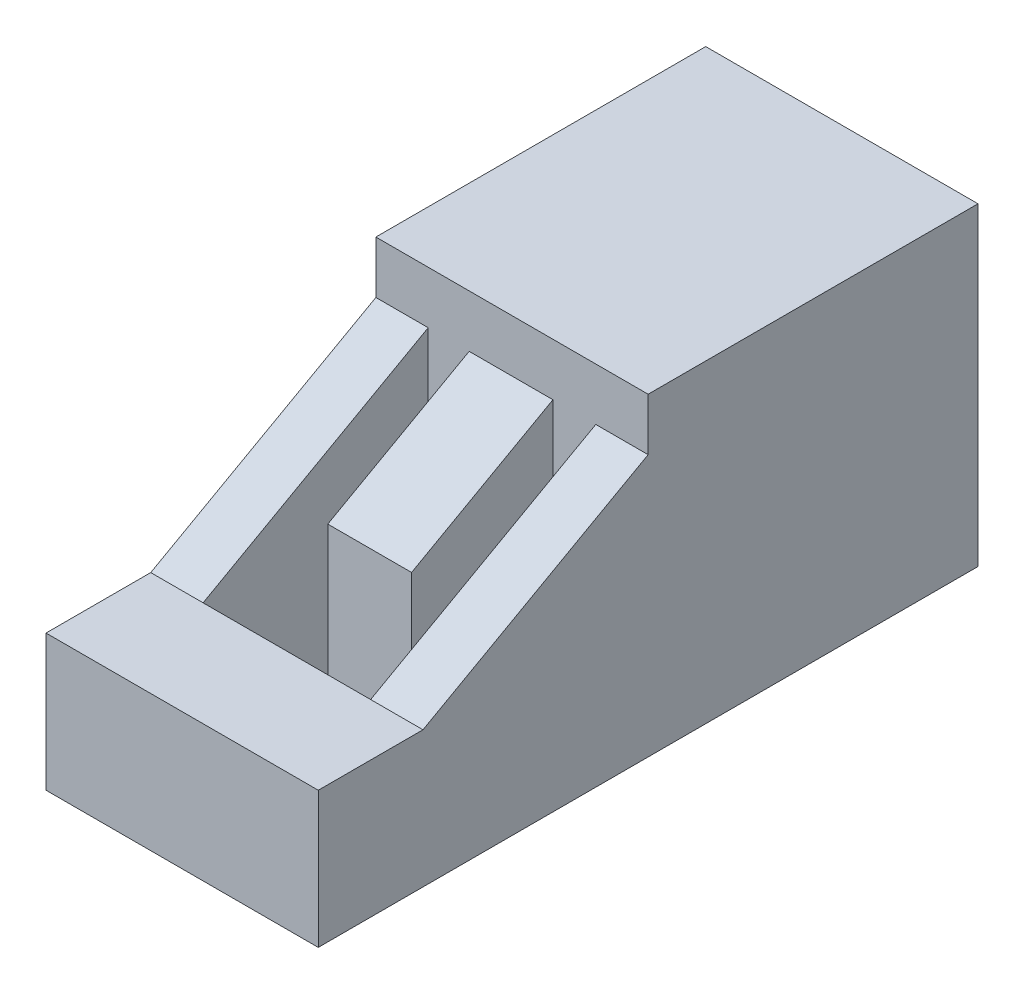
ISO-10303-21;
HEADER;
FILE_DESCRIPTION(('STEP AP214'),'2;1');
FILE_NAME('part.step','',(''),(''),'','','');
FILE_SCHEMA(('AUTOMOTIVE_DESIGN { 1 0 10303 214 1 1 1 1 }'));
ENDSEC;
DATA;
#1=APPLICATION_CONTEXT('core data for automotive mechanical design processes');
#2=APPLICATION_PROTOCOL_DEFINITION('international standard','automotive_design',2000,#1);
#3=PRODUCT_CONTEXT('',#1,'mechanical');
#4=PRODUCT('Part','Part','',(#3));
#5=PRODUCT_RELATED_PRODUCT_CATEGORY('part','',(#4));
#6=PRODUCT_DEFINITION_FORMATION('','',#4);
#7=PRODUCT_DEFINITION_CONTEXT('part definition',#1,'design');
#8=PRODUCT_DEFINITION('design','',#6,#7);
#9=PRODUCT_DEFINITION_SHAPE('','',#8);
#10=(LENGTH_UNIT() NAMED_UNIT(*) SI_UNIT(.MILLI.,.METRE.));
#11=(NAMED_UNIT(*) PLANE_ANGLE_UNIT() SI_UNIT($,.RADIAN.));
#12=(NAMED_UNIT(*) SI_UNIT($,.STERADIAN.) SOLID_ANGLE_UNIT());
#13=UNCERTAINTY_MEASURE_WITH_UNIT(LENGTH_MEASURE(1.E-05),#10,'distance_accuracy_value','');
#14=(GEOMETRIC_REPRESENTATION_CONTEXT(3) GLOBAL_UNCERTAINTY_ASSIGNED_CONTEXT((#13)) GLOBAL_UNIT_ASSIGNED_CONTEXT((#10,
#11,#12)) REPRESENTATION_CONTEXT('',''));
#15=CARTESIAN_POINT('',(0.,0.,0.));
#16=DIRECTION('',(0.,0.,1.));
#17=DIRECTION('',(1.,0.,0.));
#18=AXIS2_PLACEMENT_3D('',#15,#16,#17);
#19=CARTESIAN_POINT('',(26.,-15.,31.5));
#20=DIRECTION('',(0.,1.,0.));
#21=DIRECTION('',(0.,0.,1.));
#22=AXIS2_PLACEMENT_3D('',#19,#20,#21);
#23=PLANE('',#22);
#24=DIRECTION('',(0.,0.,1.));
#25=VECTOR('',#24,1.);
#26=CARTESIAN_POINT('',(8.90839032863548,-15.,31.5));
#27=LINE('',#26,#25);
#28=CARTESIAN_POINT('',(8.90839032863548,-15.,0.));
#29=VERTEX_POINT('',#28);
#30=CARTESIAN_POINT('',(8.90839032863548,-15.,13.5));
#31=VERTEX_POINT('',#30);
#32=EDGE_CURVE('E171',#29,#31,#27,.T.);
#33=ORIENTED_EDGE('',*,*,#32,.F.);
#34=DIRECTION('',(1.,0.,0.));
#35=VECTOR('',#34,1.);
#36=CARTESIAN_POINT('',(26.,-15.,0.));
#37=LINE('',#36,#35);
#38=CARTESIAN_POINT('',(4.99999999999999,-15.,0.));
#39=VERTEX_POINT('',#38);
#40=EDGE_CURVE('E180',#39,#29,#37,.T.);
#41=ORIENTED_EDGE('',*,*,#40,.F.);
#42=DIRECTION('',(0.,0.,1.));
#43=VECTOR('',#42,1.);
#44=CARTESIAN_POINT('',(4.99999999999999,-15.,31.5));
#45=LINE('',#44,#43);
#46=CARTESIAN_POINT('',(4.99999999999999,-15.,21.5));
#47=VERTEX_POINT('',#46);
#48=EDGE_CURVE('E179',#39,#47,#45,.T.);
#49=ORIENTED_EDGE('',*,*,#48,.T.);
#50=DIRECTION('',(1.,0.,0.));
#51=VECTOR('',#50,1.);
#52=CARTESIAN_POINT('',(26.,-15.,21.5));
#53=LINE('',#52,#51);
#54=CARTESIAN_POINT('',(21.,-15.,21.5));
#55=VERTEX_POINT('',#54);
#56=EDGE_CURVE('E185',#47,#55,#53,.T.);
#57=ORIENTED_EDGE('',*,*,#56,.T.);
#58=DIRECTION('',(0.,0.,1.));
#59=VECTOR('',#58,1.);
#60=CARTESIAN_POINT('',(21.,-15.,31.5));
#61=LINE('',#60,#59);
#62=CARTESIAN_POINT('',(21.,-15.,0.));
#63=VERTEX_POINT('',#62);
#64=EDGE_CURVE('E183',#63,#55,#61,.T.);
#65=ORIENTED_EDGE('',*,*,#64,.F.);
#66=DIRECTION('',(1.,0.,0.));
#67=VECTOR('',#66,1.);
#68=CARTESIAN_POINT('',(26.,-15.,0.));
#69=LINE('',#68,#67);
#70=CARTESIAN_POINT('',(16.9083903286355,-15.,0.));
#71=VERTEX_POINT('',#70);
#72=EDGE_CURVE('E190',#71,#63,#69,.T.);
#73=ORIENTED_EDGE('',*,*,#72,.F.);
#74=DIRECTION('',(0.,0.,1.));
#75=VECTOR('',#74,1.);
#76=CARTESIAN_POINT('',(16.9083903286355,-15.,31.5));
#77=LINE('',#76,#75);
#78=CARTESIAN_POINT('',(16.9083903286355,-15.,13.5));
#79=VERTEX_POINT('',#78);
#80=EDGE_CURVE('E163',#71,#79,#77,.T.);
#81=ORIENTED_EDGE('',*,*,#80,.T.);
#82=DIRECTION('',(1.,0.,0.));
#83=VECTOR('',#82,1.);
#84=CARTESIAN_POINT('',(26.,-15.,13.5));
#85=LINE('',#84,#83);
#86=EDGE_CURVE('E175',#31,#79,#85,.T.);
#87=ORIENTED_EDGE('',*,*,#86,.F.);
#88=EDGE_LOOP('',(#33,#41,#49,#57,#65,#73,#81,#87));
#89=FACE_BOUND('',#88,.T.);
#90=DIRECTION('',(0.,0.,-1.));
#91=VECTOR('',#90,1.);
#92=CARTESIAN_POINT('',(0.,-15.,31.5));
#93=LINE('',#92,#91);
#94=CARTESIAN_POINT('',(0.,-15.,31.5));
#95=VERTEX_POINT('',#94);
#96=CARTESIAN_POINT('',(0.,-15.,-31.5));
#97=VERTEX_POINT('',#96);
#98=EDGE_CURVE('E224',#95,#97,#93,.T.);
#99=ORIENTED_EDGE('',*,*,#98,.T.);
#100=DIRECTION('',(-1.,0.,0.));
#101=VECTOR('',#100,1.);
#102=CARTESIAN_POINT('',(26.,-15.,-31.5));
#103=LINE('',#102,#101);
#104=CARTESIAN_POINT('',(26.,-15.,-31.5));
#105=VERTEX_POINT('',#104);
#106=EDGE_CURVE('E226',#105,#97,#103,.T.);
#107=ORIENTED_EDGE('',*,*,#106,.F.);
#108=DIRECTION('',(0.,0.,-1.));
#109=VECTOR('',#108,1.);
#110=CARTESIAN_POINT('',(26.,-15.,31.5));
#111=LINE('',#110,#109);
#112=CARTESIAN_POINT('',(26.,-15.,31.5));
#113=VERTEX_POINT('',#112);
#114=EDGE_CURVE('E228',#113,#105,#111,.T.);
#115=ORIENTED_EDGE('',*,*,#114,.F.);
#116=DIRECTION('',(-1.,0.,0.));
#117=VECTOR('',#116,1.);
#118=CARTESIAN_POINT('',(26.,-15.,31.5));
#119=LINE('',#118,#117);
#120=EDGE_CURVE('E242',#113,#95,#119,.T.);
#121=ORIENTED_EDGE('',*,*,#120,.T.);
#122=EDGE_LOOP('',(#99,#107,#115,#121));
#123=FACE_BOUND('',#122,.T.);
#124=ADVANCED_FACE('F41',(#89,#123),#23,.F.);
#125=CARTESIAN_POINT('',(0.,7.62474226804124,4.25567010309278));
#126=DIRECTION('',(0.,-0.873197702014912,-0.487366159264137));
#127=DIRECTION('',(0.,0.487366159264137,-0.873197702014913));
#128=AXIS2_PLACEMENT_3D('',#125,#126,#127);
#129=PLANE('',#128);
#130=DIRECTION('',(0.,0.487366159264137,-0.873197702014913));
#131=VECTOR('',#130,1.);
#132=CARTESIAN_POINT('',(21.,7.62474226804124,4.25567010309278));
#133=LINE('',#132,#131);
#134=CARTESIAN_POINT('',(21.,-2.,21.5));
#135=VERTEX_POINT('',#134);
#136=CARTESIAN_POINT('',(21.,9.99999999999999,0.));
#137=VERTEX_POINT('',#136);
#138=EDGE_CURVE('E11',#135,#137,#133,.T.);
#139=ORIENTED_EDGE('',*,*,#138,.F.);
#140=DIRECTION('',(1.,0.,0.));
#141=VECTOR('',#140,1.);
#142=CARTESIAN_POINT('',(0.,-2.,21.5));
#143=LINE('',#142,#141);
#144=CARTESIAN_POINT('',(26.,-2.,21.5));
#145=VERTEX_POINT('',#144);
#146=EDGE_CURVE('E200',#135,#145,#143,.T.);
#147=ORIENTED_EDGE('',*,*,#146,.T.);
#148=DIRECTION('',(0.,0.487366159264137,-0.873197702014912));
#149=VECTOR('',#148,1.);
#150=CARTESIAN_POINT('',(26.,7.62474226804124,4.25567010309278));
#151=LINE('',#150,#149);
#152=CARTESIAN_POINT('',(26.,10.,0.));
#153=VERTEX_POINT('',#152);
#154=EDGE_CURVE('E205',#145,#153,#151,.T.);
#155=ORIENTED_EDGE('',*,*,#154,.T.);
#156=DIRECTION('',(1.,0.,0.));
#157=VECTOR('',#156,1.);
#158=CARTESIAN_POINT('',(0.,10.,0.));
#159=LINE('',#158,#157);
#160=EDGE_CURVE('E212',#137,#153,#159,.T.);
#161=ORIENTED_EDGE('',*,*,#160,.F.);
#162=EDGE_LOOP('',(#139,#147,#155,#161));
#163=FACE_BOUND('',#162,.T.);
#164=ADVANCED_FACE('F286',(#163),#129,.F.);
#165=CARTESIAN_POINT('',(26.,15.,-31.5));
#166=DIRECTION('',(0.,0.,1.));
#167=DIRECTION('',(1.,0.,0.));
#168=AXIS2_PLACEMENT_3D('',#165,#166,#167);
#169=PLANE('',#168);
#170=DIRECTION('',(0.,1.,0.));
#171=VECTOR('',#170,1.);
#172=CARTESIAN_POINT('',(0.,15.,-31.5));
#173=LINE('',#172,#171);
#174=CARTESIAN_POINT('',(0.,15.,-31.5));
#175=VERTEX_POINT('',#174);
#176=EDGE_CURVE('E208',#97,#175,#173,.T.);
#177=ORIENTED_EDGE('',*,*,#176,.T.);
#178=DIRECTION('',(-1.,0.,0.));
#179=VECTOR('',#178,1.);
#180=CARTESIAN_POINT('',(26.,15.,-31.5));
#181=LINE('',#180,#179);
#182=CARTESIAN_POINT('',(26.,15.,-31.5));
#183=VERTEX_POINT('',#182);
#184=EDGE_CURVE('E244',#183,#175,#181,.T.);
#185=ORIENTED_EDGE('',*,*,#184,.F.);
#186=DIRECTION('',(0.,1.,0.));
#187=VECTOR('',#186,1.);
#188=CARTESIAN_POINT('',(26.,15.,-31.5));
#189=LINE('',#188,#187);
#190=EDGE_CURVE('E218',#105,#183,#189,.T.);
#191=ORIENTED_EDGE('',*,*,#190,.F.);
#192=ORIENTED_EDGE('',*,*,#106,.T.);
#193=EDGE_LOOP('',(#177,#185,#191,#192));
#194=FACE_BOUND('',#193,.T.);
#195=ADVANCED_FACE('F43',(#194),#169,.F.);
#196=CARTESIAN_POINT('',(26.,15.,31.5));
#197=DIRECTION('',(0.,-1.,0.));
#198=DIRECTION('',(0.,0.,-1.));
#199=AXIS2_PLACEMENT_3D('',#196,#197,#198);
#200=PLANE('',#199);
#201=DIRECTION('',(1.,0.,0.));
#202=VECTOR('',#201,1.);
#203=CARTESIAN_POINT('',(0.,15.,0.));
#204=LINE('',#203,#202);
#205=CARTESIAN_POINT('',(0.,15.,0.));
#206=VERTEX_POINT('',#205);
#207=CARTESIAN_POINT('',(26.,15.,0.));
#208=VERTEX_POINT('',#207);
#209=EDGE_CURVE('E207',#206,#208,#204,.T.);
#210=ORIENTED_EDGE('',*,*,#209,.T.);
#211=DIRECTION('',(0.,0.,1.));
#212=VECTOR('',#211,1.);
#213=CARTESIAN_POINT('',(26.,15.,31.5));
#214=LINE('',#213,#212);
#215=EDGE_CURVE('E225',#183,#208,#214,.T.);
#216=ORIENTED_EDGE('',*,*,#215,.F.);
#217=ORIENTED_EDGE('',*,*,#184,.T.);
#218=DIRECTION('',(0.,0.,1.));
#219=VECTOR('',#218,1.);
#220=CARTESIAN_POINT('',(0.,15.,31.5));
#221=LINE('',#220,#219);
#222=EDGE_CURVE('E233',#175,#206,#221,.T.);
#223=ORIENTED_EDGE('',*,*,#222,.T.);
#224=EDGE_LOOP('',(#210,#216,#217,#223));
#225=FACE_BOUND('',#224,.T.);
#226=ADVANCED_FACE('F266',(#225),#200,.F.);
#227=CARTESIAN_POINT('',(26.,15.,31.5));
#228=DIRECTION('',(0.,0.,-1.));
#229=DIRECTION('',(0.,1.,0.));
#230=AXIS2_PLACEMENT_3D('',#227,#228,#229);
#231=PLANE('',#230);
#232=DIRECTION('',(0.,-1.,0.));
#233=VECTOR('',#232,1.);
#234=CARTESIAN_POINT('',(26.,15.,31.5));
#235=LINE('',#234,#233);
#236=CARTESIAN_POINT('',(26.,-2.,31.5));
#237=VERTEX_POINT('',#236);
#238=EDGE_CURVE('E227',#237,#113,#235,.T.);
#239=ORIENTED_EDGE('',*,*,#238,.F.);
#240=DIRECTION('',(1.,0.,0.));
#241=VECTOR('',#240,1.);
#242=CARTESIAN_POINT('',(0.,-2.,31.5));
#243=LINE('',#242,#241);
#244=CARTESIAN_POINT('',(0.,-2.,31.5));
#245=VERTEX_POINT('',#244);
#246=EDGE_CURVE('E206',#245,#237,#243,.T.);
#247=ORIENTED_EDGE('',*,*,#246,.F.);
#248=DIRECTION('',(0.,-1.,0.));
#249=VECTOR('',#248,1.);
#250=CARTESIAN_POINT('',(0.,15.,31.5));
#251=LINE('',#250,#249);
#252=EDGE_CURVE('E237',#245,#95,#251,.T.);
#253=ORIENTED_EDGE('',*,*,#252,.T.);
#254=ORIENTED_EDGE('',*,*,#120,.F.);
#255=EDGE_LOOP('',(#239,#247,#253,#254));
#256=FACE_BOUND('',#255,.T.);
#257=ADVANCED_FACE('F280',(#256),#231,.F.);
#258=CARTESIAN_POINT('',(26.,0.,0.));
#259=DIRECTION('',(1.,0.,0.));
#260=DIRECTION('',(0.,0.,-1.));
#261=AXIS2_PLACEMENT_3D('',#258,#259,#260);
#262=PLANE('',#261);
#263=DIRECTION('',(0.,0.,-1.));
#264=VECTOR('',#263,1.);
#265=CARTESIAN_POINT('',(26.,-2.,0.));
#266=LINE('',#265,#264);
#267=EDGE_CURVE('E189',#237,#145,#266,.T.);
#268=ORIENTED_EDGE('',*,*,#267,.F.);
#269=ORIENTED_EDGE('',*,*,#238,.T.);
#270=ORIENTED_EDGE('',*,*,#114,.T.);
#271=ORIENTED_EDGE('',*,*,#190,.T.);
#272=ORIENTED_EDGE('',*,*,#215,.T.);
#273=DIRECTION('',(0.,1.,0.));
#274=VECTOR('',#273,1.);
#275=CARTESIAN_POINT('',(26.,0.,0.));
#276=LINE('',#275,#274);
#277=EDGE_CURVE('E194',#153,#208,#276,.T.);
#278=ORIENTED_EDGE('',*,*,#277,.F.);
#279=ORIENTED_EDGE('',*,*,#154,.F.);
#280=EDGE_LOOP('',(#268,#269,#270,#271,#272,#278,#279));
#281=FACE_BOUND('',#280,.T.);
#282=ADVANCED_FACE('F281',(#281),#262,.T.);
#283=CARTESIAN_POINT('',(0.,0.,0.));
#284=DIRECTION('',(1.,0.,0.));
#285=DIRECTION('',(0.,0.,-1.));
#286=AXIS2_PLACEMENT_3D('',#283,#284,#285);
#287=PLANE('',#286);
#288=ORIENTED_EDGE('',*,*,#252,.F.);
#289=DIRECTION('',(0.,0.,-1.));
#290=VECTOR('',#289,1.);
#291=CARTESIAN_POINT('',(0.,-2.,0.));
#292=LINE('',#291,#290);
#293=CARTESIAN_POINT('',(0.,-2.,21.5));
#294=VERTEX_POINT('',#293);
#295=EDGE_CURVE('E186',#245,#294,#292,.T.);
#296=ORIENTED_EDGE('',*,*,#295,.T.);
#297=DIRECTION('',(0.,0.487366159264137,-0.873197702014912));
#298=VECTOR('',#297,1.);
#299=CARTESIAN_POINT('',(0.,7.62474226804124,4.25567010309278));
#300=LINE('',#299,#298);
#301=CARTESIAN_POINT('',(0.,10.,0.));
#302=VERTEX_POINT('',#301);
#303=EDGE_CURVE('E193',#294,#302,#300,.T.);
#304=ORIENTED_EDGE('',*,*,#303,.T.);
#305=DIRECTION('',(0.,1.,0.));
#306=VECTOR('',#305,1.);
#307=CARTESIAN_POINT('',(0.,0.,0.));
#308=LINE('',#307,#306);
#309=EDGE_CURVE('E198',#302,#206,#308,.T.);
#310=ORIENTED_EDGE('',*,*,#309,.T.);
#311=ORIENTED_EDGE('',*,*,#222,.F.);
#312=ORIENTED_EDGE('',*,*,#176,.F.);
#313=ORIENTED_EDGE('',*,*,#98,.F.);
#314=EDGE_LOOP('',(#288,#296,#304,#310,#311,#312,#313));
#315=FACE_BOUND('',#314,.T.);
#316=ADVANCED_FACE('F263',(#315),#287,.F.);
#317=CARTESIAN_POINT('',(0.,-2.,0.));
#318=DIRECTION('',(0.,-1.,0.));
#319=DIRECTION('',(0.,0.,-1.));
#320=AXIS2_PLACEMENT_3D('',#317,#318,#319);
#321=PLANE('',#320);
#322=ORIENTED_EDGE('',*,*,#267,.T.);
#323=ORIENTED_EDGE('',*,*,#146,.F.);
#324=CARTESIAN_POINT('',(4.99999999999999,-2.00000000000001,21.5));
#325=VERTEX_POINT('',#324);
#326=EDGE_CURVE('E217',#325,#135,#143,.T.);
#327=ORIENTED_EDGE('',*,*,#326,.F.);
#328=EDGE_CURVE('E214',#294,#325,#143,.T.);
#329=ORIENTED_EDGE('',*,*,#328,.F.);
#330=ORIENTED_EDGE('',*,*,#295,.F.);
#331=ORIENTED_EDGE('',*,*,#246,.T.);
#332=EDGE_LOOP('',(#322,#323,#327,#329,#330,#331));
#333=FACE_BOUND('',#332,.T.);
#334=ADVANCED_FACE('F282',(#333),#321,.F.);
#335=CARTESIAN_POINT('',(0.,0.,0.));
#336=DIRECTION('',(0.,0.,-1.));
#337=DIRECTION('',(-1.,0.,0.));
#338=AXIS2_PLACEMENT_3D('',#335,#336,#337);
#339=PLANE('',#338);
#340=ORIENTED_EDGE('',*,*,#277,.T.);
#341=ORIENTED_EDGE('',*,*,#209,.F.);
#342=ORIENTED_EDGE('',*,*,#309,.F.);
#343=CARTESIAN_POINT('',(4.99999999999999,10.,0.));
#344=VERTEX_POINT('',#343);
#345=EDGE_CURVE('E211',#302,#344,#159,.T.);
#346=ORIENTED_EDGE('',*,*,#345,.T.);
#347=DIRECTION('',(0.,1.,0.));
#348=VECTOR('',#347,1.);
#349=CARTESIAN_POINT('',(4.99999999999999,-29.,0.));
#350=LINE('',#349,#348);
#351=EDGE_CURVE('E254',#39,#344,#350,.T.);
#352=ORIENTED_EDGE('',*,*,#351,.F.);
#353=ORIENTED_EDGE('',*,*,#40,.T.);
#354=DIRECTION('',(0.,1.,0.));
#355=VECTOR('',#354,1.);
#356=CARTESIAN_POINT('',(8.90839032863548,-29.,0.));
#357=LINE('',#356,#355);
#358=CARTESIAN_POINT('',(8.90839032863548,10.,0.));
#359=VERTEX_POINT('',#358);
#360=EDGE_CURVE('E154',#29,#359,#357,.T.);
#361=ORIENTED_EDGE('',*,*,#360,.T.);
#362=DIRECTION('',(1.,0.,0.));
#363=VECTOR('',#362,1.);
#364=CARTESIAN_POINT('',(-13.0916096713645,10.,0.));
#365=LINE('',#364,#363);
#366=CARTESIAN_POINT('',(16.9083903286355,10.,0.));
#367=VERTEX_POINT('',#366);
#368=EDGE_CURVE('E146',#359,#367,#365,.T.);
#369=ORIENTED_EDGE('',*,*,#368,.T.);
#370=DIRECTION('',(0.,1.,0.));
#371=VECTOR('',#370,1.);
#372=CARTESIAN_POINT('',(16.9083903286355,-29.,0.));
#373=LINE('',#372,#371);
#374=EDGE_CURVE('E155',#71,#367,#373,.T.);
#375=ORIENTED_EDGE('',*,*,#374,.F.);
#376=ORIENTED_EDGE('',*,*,#72,.T.);
#377=DIRECTION('',(0.,1.,0.));
#378=VECTOR('',#377,1.);
#379=CARTESIAN_POINT('',(21.,-29.,0.));
#380=LINE('',#379,#378);
#381=EDGE_CURVE('E173',#63,#137,#380,.T.);
#382=ORIENTED_EDGE('',*,*,#381,.T.);
#383=ORIENTED_EDGE('',*,*,#160,.T.);
#384=EDGE_LOOP('',(#340,#341,#342,#346,#352,#353,#361,#369,#375,#376,#382,#383));
#385=FACE_BOUND('',#384,.T.);
#386=ADVANCED_FACE('F147',(#385),#339,.F.);
#387=DIRECTION('',(0.,0.487366159264137,-0.873197702014913));
#388=VECTOR('',#387,1.);
#389=CARTESIAN_POINT('',(4.99999999999999,7.62474226804124,4.25567010309278));
#390=LINE('',#389,#388);
#391=EDGE_CURVE('E47',#325,#344,#390,.T.);
#392=ORIENTED_EDGE('',*,*,#391,.T.);
#393=ORIENTED_EDGE('',*,*,#345,.F.);
#394=ORIENTED_EDGE('',*,*,#303,.F.);
#395=ORIENTED_EDGE('',*,*,#328,.T.);
#396=EDGE_LOOP('',(#392,#393,#394,#395));
#397=FACE_BOUND('',#396,.T.);
#398=ADVANCED_FACE('F249',(#397),#129,.F.);
#399=CARTESIAN_POINT('',(21.,-29.,0.));
#400=DIRECTION('',(-1.,0.,0.));
#401=DIRECTION('',(0.,0.,1.));
#402=AXIS2_PLACEMENT_3D('',#399,#400,#401);
#403=PLANE('',#402);
#404=ORIENTED_EDGE('',*,*,#64,.T.);
#405=DIRECTION('',(0.,1.,0.));
#406=VECTOR('',#405,1.);
#407=CARTESIAN_POINT('',(21.,-29.,21.5));
#408=LINE('',#407,#406);
#409=EDGE_CURVE('E297',#55,#135,#408,.T.);
#410=ORIENTED_EDGE('',*,*,#409,.T.);
#411=ORIENTED_EDGE('',*,*,#138,.T.);
#412=ORIENTED_EDGE('',*,*,#381,.F.);
#413=EDGE_LOOP('',(#404,#410,#411,#412));
#414=FACE_BOUND('',#413,.T.);
#415=ADVANCED_FACE('F298',(#414),#403,.T.);
#416=CARTESIAN_POINT('',(0.,-29.,21.5));
#417=DIRECTION('',(0.,0.,1.));
#418=DIRECTION('',(1.,0.,0.));
#419=AXIS2_PLACEMENT_3D('',#416,#417,#418);
#420=PLANE('',#419);
#421=DIRECTION('',(0.,1.,0.));
#422=VECTOR('',#421,1.);
#423=CARTESIAN_POINT('',(4.99999999999999,-29.,21.5));
#424=LINE('',#423,#422);
#425=EDGE_CURVE('E256',#47,#325,#424,.T.);
#426=ORIENTED_EDGE('',*,*,#425,.T.);
#427=ORIENTED_EDGE('',*,*,#326,.T.);
#428=ORIENTED_EDGE('',*,*,#409,.F.);
#429=ORIENTED_EDGE('',*,*,#56,.F.);
#430=EDGE_LOOP('',(#426,#427,#428,#429));
#431=FACE_BOUND('',#430,.T.);
#432=ADVANCED_FACE('F293',(#431),#420,.F.);
#433=CARTESIAN_POINT('',(4.99999999999999,-29.,0.));
#434=DIRECTION('',(-1.,0.,0.));
#435=DIRECTION('',(0.,0.,1.));
#436=AXIS2_PLACEMENT_3D('',#433,#434,#435);
#437=PLANE('',#436);
#438=ORIENTED_EDGE('',*,*,#351,.T.);
#439=ORIENTED_EDGE('',*,*,#391,.F.);
#440=ORIENTED_EDGE('',*,*,#425,.F.);
#441=ORIENTED_EDGE('',*,*,#48,.F.);
#442=EDGE_LOOP('',(#438,#439,#440,#441));
#443=FACE_BOUND('',#442,.T.);
#444=ADVANCED_FACE('F258',(#443),#437,.F.);
#445=CARTESIAN_POINT('',(8.90839032863548,-29.,0.));
#446=DIRECTION('',(-1.,0.,0.));
#447=DIRECTION('',(0.,0.,1.));
#448=AXIS2_PLACEMENT_3D('',#445,#446,#447);
#449=PLANE('',#448);
#450=DIRECTION('',(0.,-0.487366159264137,0.873197702014913));
#451=VECTOR('',#450,1.);
#452=CARTESIAN_POINT('',(8.90839032863548,0.736494845360827,16.5971134020619));
#453=LINE('',#452,#451);
#454=CARTESIAN_POINT('',(8.90839032863548,2.46511627906977,13.5));
#455=VERTEX_POINT('',#454);
#456=EDGE_CURVE('E160',#359,#455,#453,.T.);
#457=ORIENTED_EDGE('',*,*,#456,.F.);
#458=ORIENTED_EDGE('',*,*,#360,.F.);
#459=ORIENTED_EDGE('',*,*,#32,.T.);
#460=DIRECTION('',(0.,1.,0.));
#461=VECTOR('',#460,1.);
#462=CARTESIAN_POINT('',(8.90839032863548,-29.,13.5));
#463=LINE('',#462,#461);
#464=EDGE_CURVE('E167',#31,#455,#463,.T.);
#465=ORIENTED_EDGE('',*,*,#464,.T.);
#466=EDGE_LOOP('',(#457,#458,#459,#465));
#467=FACE_BOUND('',#466,.T.);
#468=ADVANCED_FACE('F310',(#467),#449,.T.);
#469=CARTESIAN_POINT('',(0.,-29.,13.5));
#470=DIRECTION('',(0.,0.,1.));
#471=DIRECTION('',(1.,0.,0.));
#472=AXIS2_PLACEMENT_3D('',#469,#470,#471);
#473=PLANE('',#472);
#474=DIRECTION('',(1.,0.,0.));
#475=VECTOR('',#474,1.);
#476=CARTESIAN_POINT('',(-13.0916096713645,2.46511627906977,13.5));
#477=LINE('',#476,#475);
#478=CARTESIAN_POINT('',(16.9083903286355,2.46511627906976,13.5));
#479=VERTEX_POINT('',#478);
#480=EDGE_CURVE('E57',#455,#479,#477,.T.);
#481=ORIENTED_EDGE('',*,*,#480,.F.);
#482=ORIENTED_EDGE('',*,*,#464,.F.);
#483=ORIENTED_EDGE('',*,*,#86,.T.);
#484=DIRECTION('',(0.,1.,0.));
#485=VECTOR('',#484,1.);
#486=CARTESIAN_POINT('',(16.9083903286355,-29.,13.5));
#487=LINE('',#486,#485);
#488=EDGE_CURVE('E63',#79,#479,#487,.T.);
#489=ORIENTED_EDGE('',*,*,#488,.T.);
#490=EDGE_LOOP('',(#481,#482,#483,#489));
#491=FACE_BOUND('',#490,.T.);
#492=ADVANCED_FACE('F311',(#491),#473,.T.);
#493=CARTESIAN_POINT('',(16.9083903286355,-29.,0.));
#494=DIRECTION('',(-1.,0.,0.));
#495=DIRECTION('',(0.,0.,1.));
#496=AXIS2_PLACEMENT_3D('',#493,#494,#495);
#497=PLANE('',#496);
#498=ORIENTED_EDGE('',*,*,#374,.T.);
#499=DIRECTION('',(0.,0.487366159264137,-0.873197702014912));
#500=VECTOR('',#499,1.);
#501=CARTESIAN_POINT('',(16.9083903286355,10.,0.));
#502=LINE('',#501,#500);
#503=EDGE_CURVE('E157',#479,#367,#502,.T.);
#504=ORIENTED_EDGE('',*,*,#503,.F.);
#505=ORIENTED_EDGE('',*,*,#488,.F.);
#506=ORIENTED_EDGE('',*,*,#80,.F.);
#507=EDGE_LOOP('',(#498,#504,#505,#506));
#508=FACE_BOUND('',#507,.T.);
#509=ADVANCED_FACE('F165',(#508),#497,.F.);
#510=CARTESIAN_POINT('',(-13.0916096713645,10.,0.));
#511=DIRECTION('',(0.,-0.873197702014913,-0.487366159264137));
#512=DIRECTION('',(0.,0.487366159264137,-0.873197702014913));
#513=AXIS2_PLACEMENT_3D('',#510,#511,#512);
#514=PLANE('',#513);
#515=ORIENTED_EDGE('',*,*,#456,.T.);
#516=ORIENTED_EDGE('',*,*,#480,.T.);
#517=ORIENTED_EDGE('',*,*,#503,.T.);
#518=ORIENTED_EDGE('',*,*,#368,.F.);
#519=EDGE_LOOP('',(#515,#516,#517,#518));
#520=FACE_BOUND('',#519,.T.);
#521=ADVANCED_FACE('F159',(#520),#514,.F.);
#522=CLOSED_SHELL('',(#124,#164,#195,#226,#257,#282,#316,#334,#386,#398,#415,#432,#444,#468,
#492,#509,#521));
#523=MANIFOLD_SOLID_BREP('B2',#522);
#524=ADVANCED_BREP_SHAPE_REPRESENTATION('',(#18,#523),#14);
#525=SHAPE_DEFINITION_REPRESENTATION(#9,#524);
ENDSEC;
END-ISO-10303-21;
